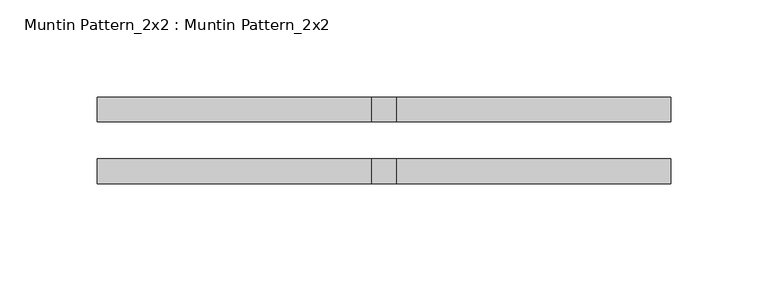
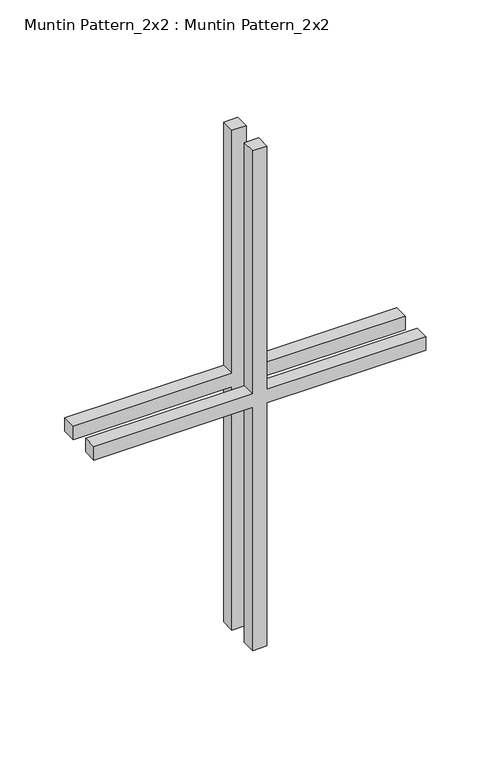
"""IFC4 building model written with IfcOpenShell, lengths in millimetres: proxy geometry, Muntin Pattern_2x2 : Muntin Pattern_2x2."""

from ifc_helpers import new_model, si_unit, frame, origin, place, context, project, spatial, polyline, outline, extrude, source, transform, mapped, element, save


def muntin_pattern_2x2_muntin_pattern_2x2_78ce0566(model_context):
    return source(origin(), model_context, "Body", "SweptSolid", [
        extrude(outline(polyline([(241.3, -6.35), (241.3, -147.6375), (228.6, -147.6375), (228.6, -6.35), (0.0, -6.35), (0.0, 6.35), (228.6, 6.35), (228.6, 147.6375), (241.3, 147.6375), (241.3, 6.35), (469.9, 6.35), (469.9, -6.35), (241.3, -6.35)])), frame((0.0, 9.525, 0.0), z_axis=(0.0, 1.0, 0.0), x_axis=(0.0, 0.0, 1.0)), (0.0, 0.0, 1.0), 12.7),
        extrude(outline(polyline([(241.3, -6.35), (241.3, -147.6375), (228.6, -147.6375), (228.6, -6.35), (0.0, -6.35), (0.0, 6.35), (228.6, 6.35), (228.6, 147.6375), (241.3, 147.6375), (241.3, 6.35), (469.9, 6.35), (469.9, -6.35), (241.3, -6.35)])), frame((0.0, -22.225, 0.0), z_axis=(0.0, 1.0, 0.0), x_axis=(0.0, 0.0, 1.0)), (0.0, 0.0, 1.0), 12.7),
    ])


if __name__ == "__main__":
    model = new_model("IFC4")
    model_context = context("Model", 3, world=origin())
    ifc_project = project(units=[si_unit("LENGTHUNIT", "METRE", prefix="MILLI")], contexts=[model_context])
    site = spatial("IfcSite", under=ifc_project)
    building = spatial("IfcBuilding", under=site)
    placement = place(None, origin())
    muntin_pattern_2x2_muntin_pattern_2x2_shape = muntin_pattern_2x2_muntin_pattern_2x2_78ce0566(model_context)
    element("IfcBuildingElementProxy", 1, Name="Muntin Pattern_2x2 : Muntin Pattern_2x2", ObjectType="Muntin Pattern_2x2 : Muntin Pattern_2x2", at=placement, inside=building, context=model_context, shape_type="MappedRepresentation", body=[
        mapped(muntin_pattern_2x2_muntin_pattern_2x2_shape, transform((0.0, 0.0, 0.0), x_axis=(1.0, 0.0, 0.0), y_axis=(0.0, 1.0, 0.0), z_axis=(0.0, 0.0, 1.0))),
    ])
    save(model, "model.ifc")

# Revit data of these elements
# Type "Muntin Pattern_2x2 : Muntin Pattern_2x2"
#   Width [instance default] = 4' - 0"
#   Thickness = 0' - 0 1/2"
#   Height [instance default] = 4' - 0"
#   Distance = 0' - 0 3/4"
#   Interior Material [instance default] = none
#   Exterior Material [instance default] = none
#   Default Elevation = 0
# Element 1 (IfcBuildingElementProxy, "Muntin Pattern_2x2 : Muntin Pattern_2x2")
#   Width = 0' - 11 5/8"
#   Height = 1' - 6 1/2"
#   Interior Material = Wood - Stained
#   Exterior Material = Clad - White
#   Materials on its faces: "Clad - White", "Wood - Stained"
# Materials
#   "Clad - White": class "Wood", colour RGB 242 242 238, transparency 0, Cost = 0
#   "Wood - Stained": class "Wood", colour RGB 224 178 126, transparency 0, Cost = 0
